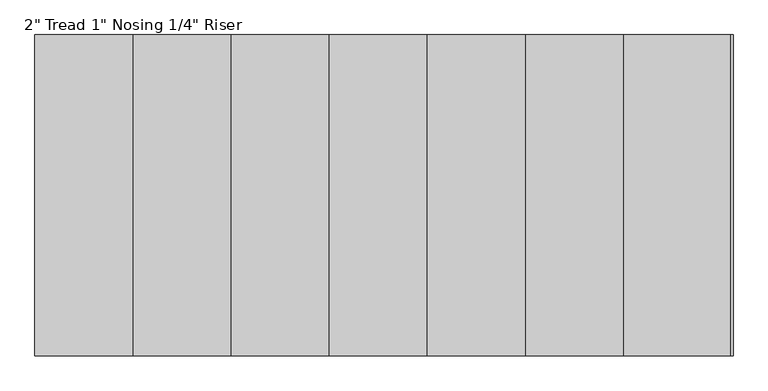
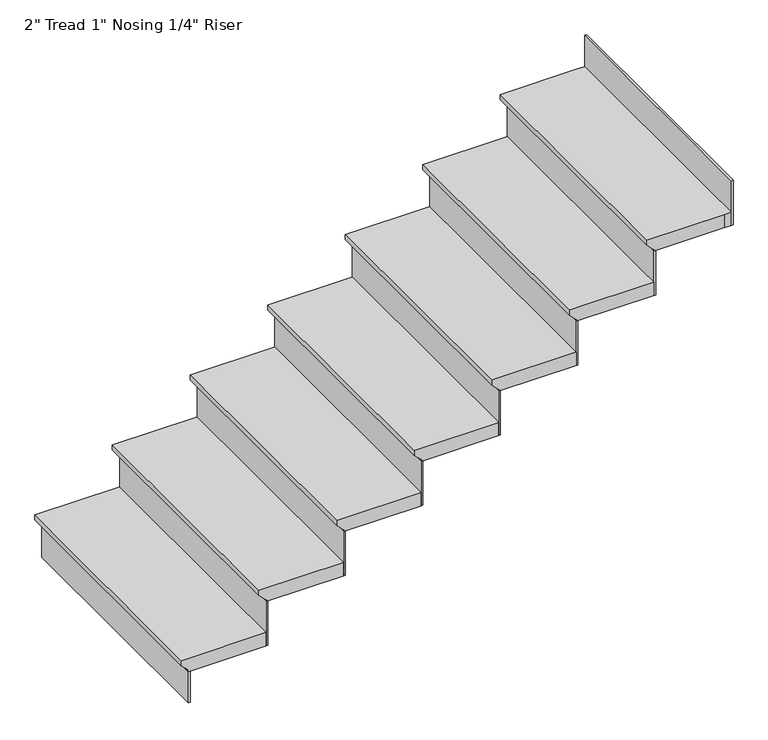
"""IFC4 building model written with IfcOpenShell, lengths in millimetres: stair flight geometry."""

from ifc_helpers import new_model, si_unit, origin, place, context, project, spatial, faceted_brep, source, transform, mapped, element, save


def stair_flight_171342da(model_context):
    return source(origin(), model_context, "Body", "Brep", [
        faceted_brep([(-1404.564062, 2339.7857363, 3503.0833333), (-1404.564062, 2339.7857363, 3522.1333333), (-1404.564062, 3254.1857363, 3522.1333333), (-1404.564062, 3254.1857363, 3503.0833333), (-1379.164062, 2339.7857363, 3477.6833333), (-1379.164062, 3254.1857363, 3477.6833333), (-1099.764062, 2339.7857363, 3522.1333333), (-1099.764062, 3254.1857363, 3522.1333333), (-1379.164062, 3254.1857363, 3471.3333333), (-1099.764062, 3254.1857363, 3471.3333333), (-1099.764062, 2339.7857363, 3471.3333333), (-1379.164062, 2339.7857363, 3471.3333333)], [[[0, 1, 2, 3]], [[4, 0, 3, 5]], [[2, 1, 6, 7]], [[8, 9, 10, 11]], [[2, 7, 9, 8, 5, 3]], [[8, 11, 4, 5]], [[6, 1, 0, 4, 11, 10]], [[7, 6, 10, 9]]]),
        faceted_brep([(-1379.164062, 2339.7857363, 3471.3333333), (-1379.164062, 2339.7857363, 3352.8), (-1372.814062, 2339.7857363, 3352.8), (-1372.814062, 2339.7857363, 3471.3333333), (-1379.164062, 3254.1857363, 3471.3333333), (-1372.814062, 3254.1857363, 3471.3333333), (-1372.814062, 3254.1857363, 3352.8), (-1379.164062, 3254.1857363, 3352.8)], [[[0, 1, 2, 3]], [[4, 5, 6, 7]], [[1, 0, 4, 7]], [[2, 1, 7, 6]], [[3, 2, 6, 5]], [[0, 3, 5, 4]]]),
        faceted_brep([(-1099.764062, 2339.7857363, 3640.6666667), (-1099.764062, 2339.7857363, 3471.3333333), (-1093.414062, 2339.7857363, 3471.3333333), (-1093.414062, 2339.7857363, 3640.6666667), (-1099.764062, 3254.1857363, 3640.6666667), (-1093.414062, 3254.1857363, 3640.6666667), (-1093.414062, 3254.1857363, 3471.3333333), (-1099.764062, 3254.1857363, 3471.3333333)], [[[0, 1, 2, 3]], [[4, 5, 6, 7]], [[1, 0, 4, 7]], [[2, 1, 7, 6]], [[3, 2, 6, 5]], [[0, 3, 5, 4]]]),
        faceted_brep([(-1125.164062, 3254.1857363, 3691.4666667), (-1125.164062, 2339.7857363, 3691.4666667), (-820.364062, 2339.7857363, 3691.4666667), (-820.364062, 3254.1857363, 3691.4666667), (-1099.764062, 3254.1857363, 3640.6666667), (-820.364062, 3254.1857363, 3640.6666667), (-820.364062, 2339.7857363, 3640.6666667), (-1099.764062, 2339.7857363, 3640.6666667), (-1099.764062, 3254.1857363, 3647.0166667), (-1125.164062, 3254.1857363, 3672.4166667), (-1099.764062, 2339.7857363, 3647.0166667), (-1125.164062, 2339.7857363, 3672.4166667)], [[[0, 1, 2, 3]], [[4, 5, 6, 7]], [[0, 3, 5, 4, 8, 9]], [[4, 7, 10, 8]], [[2, 1, 11, 10, 7, 6]], [[3, 2, 6, 5]], [[11, 1, 0, 9]], [[10, 11, 9, 8]]]),
        faceted_brep([(-820.364062, 2339.7857363, 3810.0), (-820.364062, 2339.7857363, 3640.6666667), (-814.014062, 2339.7857363, 3640.6666667), (-814.014062, 2339.7857363, 3810.0), (-820.364062, 3254.1857363, 3810.0), (-814.014062, 3254.1857363, 3810.0), (-814.014062, 3254.1857363, 3640.6666667), (-820.364062, 3254.1857363, 3640.6666667)], [[[0, 1, 2, 3]], [[4, 5, 6, 7]], [[1, 0, 4, 7]], [[2, 1, 7, 6]], [[3, 2, 6, 5]], [[0, 3, 5, 4]]]),
        faceted_brep([(-845.764062, 3254.1857363, 3860.8), (-845.764062, 2339.7857363, 3860.8), (-540.964062, 2339.7857363, 3860.8), (-540.964062, 3254.1857363, 3860.8), (-820.364062, 3254.1857363, 3810.0), (-540.964062, 3254.1857363, 3810.0), (-540.964062, 2339.7857363, 3810.0), (-820.364062, 2339.7857363, 3810.0), (-820.364062, 3254.1857363, 3816.35), (-845.764062, 3254.1857363, 3841.75), (-820.364062, 2339.7857363, 3816.35), (-845.764062, 2339.7857363, 3841.75)], [[[0, 1, 2, 3]], [[4, 5, 6, 7]], [[0, 3, 5, 4, 8, 9]], [[4, 7, 10, 8]], [[2, 1, 11, 10, 7, 6]], [[3, 2, 6, 5]], [[11, 1, 0, 9]], [[10, 11, 9, 8]]]),
        faceted_brep([(-540.964062, 2339.7857363, 3979.3333333), (-540.964062, 2339.7857363, 3810.0), (-534.614062, 2339.7857363, 3810.0), (-534.614062, 2339.7857363, 3979.3333333), (-540.964062, 3254.1857363, 3979.3333333), (-534.614062, 3254.1857363, 3979.3333333), (-534.614062, 3254.1857363, 3810.0), (-540.964062, 3254.1857363, 3810.0)], [[[0, 1, 2, 3]], [[4, 5, 6, 7]], [[1, 0, 4, 7]], [[2, 1, 7, 6]], [[3, 2, 6, 5]], [[0, 3, 5, 4]]]),
        faceted_brep([(-566.364062, 3254.1857363, 4030.1333333), (-566.364062, 2339.7857363, 4030.1333333), (-261.564062, 2339.7857363, 4030.1333333), (-261.564062, 3254.1857363, 4030.1333333), (-540.964062, 3254.1857363, 3979.3333333), (-261.564062, 3254.1857363, 3979.3333333), (-261.564062, 2339.7857363, 3979.3333333), (-540.964062, 2339.7857363, 3979.3333333), (-540.964062, 3254.1857363, 3985.6833333), (-566.364062, 3254.1857363, 4011.0833333), (-540.964062, 2339.7857363, 3985.6833333), (-566.364062, 2339.7857363, 4011.0833333)], [[[0, 1, 2, 3]], [[4, 5, 6, 7]], [[0, 3, 5, 4, 8, 9]], [[4, 7, 10, 8]], [[2, 1, 11, 10, 7, 6]], [[3, 2, 6, 5]], [[11, 1, 0, 9]], [[10, 11, 9, 8]]]),
        faceted_brep([(-261.564062, 2339.7857363, 4148.6666667), (-261.564062, 2339.7857363, 3979.3333333), (-255.214062, 2339.7857363, 3979.3333333), (-255.214062, 2339.7857363, 4148.6666667), (-261.564062, 3254.1857363, 4148.6666667), (-255.214062, 3254.1857363, 4148.6666667), (-255.214062, 3254.1857363, 3979.3333333), (-261.564062, 3254.1857363, 3979.3333333)], [[[0, 1, 2, 3]], [[4, 5, 6, 7]], [[1, 0, 4, 7]], [[2, 1, 7, 6]], [[3, 2, 6, 5]], [[0, 3, 5, 4]]]),
        faceted_brep([(-286.964062, 3254.1857363, 4199.4666667), (-286.964062, 2339.7857363, 4199.4666667), (17.835938, 2339.7857363, 4199.4666667), (17.835938, 3254.1857363, 4199.4666667), (-261.564062, 3254.1857363, 4148.6666667), (17.835938, 3254.1857363, 4148.6666667), (17.835938, 2339.7857363, 4148.6666667), (-261.564062, 2339.7857363, 4148.6666667), (-261.564062, 3254.1857363, 4155.0166667), (-286.964062, 3254.1857363, 4180.4166667), (-261.564062, 2339.7857363, 4155.0166667), (-286.964062, 2339.7857363, 4180.4166667)], [[[0, 1, 2, 3]], [[4, 5, 6, 7]], [[0, 3, 5, 4, 8, 9]], [[4, 7, 10, 8]], [[2, 1, 11, 10, 7, 6]], [[3, 2, 6, 5]], [[11, 1, 0, 9]], [[10, 11, 9, 8]]]),
        faceted_brep([(17.835938, 2339.7857363, 4318.0), (17.835938, 2339.7857363, 4148.6666667), (24.185938, 2339.7857363, 4148.6666667), (24.185938, 2339.7857363, 4318.0), (17.835938, 3254.1857363, 4318.0), (24.185938, 3254.1857363, 4318.0), (24.185938, 3254.1857363, 4148.6666667), (17.835938, 3254.1857363, 4148.6666667)], [[[0, 1, 2, 3]], [[4, 5, 6, 7]], [[1, 0, 4, 7]], [[2, 1, 7, 6]], [[3, 2, 6, 5]], [[0, 3, 5, 4]]]),
        faceted_brep([(-7.564062, 3254.1857363, 4368.8), (-7.564062, 2339.7857363, 4368.8), (297.235938, 2339.7857363, 4368.8), (297.235938, 3254.1857363, 4368.8), (17.835938, 3254.1857363, 4318.0), (297.235938, 3254.1857363, 4318.0), (297.235938, 2339.7857363, 4318.0), (17.835938, 2339.7857363, 4318.0), (17.835938, 3254.1857363, 4324.35), (-7.564062, 3254.1857363, 4349.75), (17.835938, 2339.7857363, 4324.35), (-7.564062, 2339.7857363, 4349.75)], [[[0, 1, 2, 3]], [[4, 5, 6, 7]], [[0, 3, 5, 4, 8, 9]], [[4, 7, 10, 8]], [[2, 1, 11, 10, 7, 6]], [[3, 2, 6, 5]], [[11, 1, 0, 9]], [[10, 11, 9, 8]]]),
        faceted_brep([(576.635938, 2339.7857363, 4656.6666667), (576.635938, 2339.7857363, 4487.3333333), (582.985938, 2339.7857363, 4487.3333333), (582.985938, 2339.7857363, 4656.6666667), (576.635938, 3254.1857363, 4656.6666667), (582.985938, 3254.1857363, 4656.6666667), (582.985938, 3254.1857363, 4487.3333333), (576.635938, 3254.1857363, 4487.3333333)], [[[0, 1, 2, 3]], [[4, 5, 6, 7]], [[1, 0, 4, 7]], [[2, 1, 7, 6]], [[3, 2, 6, 5]], [[0, 3, 5, 4]]]),
        faceted_brep([(297.235938, 2339.7857363, 4487.3333333), (297.235938, 2339.7857363, 4318.0), (303.585938, 2339.7857363, 4318.0), (303.585938, 2339.7857363, 4487.3333333), (297.235938, 3254.1857363, 4487.3333333), (303.585938, 3254.1857363, 4487.3333333), (303.585938, 3254.1857363, 4318.0), (297.235938, 3254.1857363, 4318.0)], [[[0, 1, 2, 3]], [[4, 5, 6, 7]], [[1, 0, 4, 7]], [[2, 1, 7, 6]], [[3, 2, 6, 5]], [[0, 3, 5, 4]]]),
        faceted_brep([(576.635938, 3254.1857363, 4538.1333333), (551.235938, 3254.1857363, 4538.1333333), (271.835938, 3254.1857363, 4538.1333333), (271.835938, 2339.7857363, 4538.1333333), (551.235938, 2339.7857363, 4538.1333333), (576.635938, 2339.7857363, 4538.1333333), (551.235938, 3254.1857363, 4487.3333333), (576.635938, 3254.1857363, 4487.3333333), (576.635938, 2339.7857363, 4487.3333333), (551.235938, 2339.7857363, 4487.3333333), (297.235938, 2339.7857363, 4487.3333333), (297.235938, 3254.1857363, 4487.3333333), (297.235938, 3254.1857363, 4493.6833333), (271.835938, 3254.1857363, 4519.0833333), (297.235938, 2339.7857363, 4493.6833333), (271.835938, 2339.7857363, 4519.0833333)], [[[0, 1, 2, 3, 4, 5]], [[6, 7, 8, 9, 10, 11]], [[1, 0, 7, 6]], [[2, 1, 6, 11, 12, 13]], [[11, 10, 14, 12]], [[4, 3, 15, 14, 10, 9]], [[5, 4, 9, 8]], [[0, 5, 8, 7]], [[15, 3, 2, 13]], [[14, 15, 13, 12]]]),
    ])


if __name__ == "__main__":
    model = new_model("IFC4")
    model_context = context("Model", 3, world=origin())
    ifc_project = project(units=[si_unit("LENGTHUNIT", "METRE", prefix="MILLI")], contexts=[model_context])
    site = spatial("IfcSite", under=ifc_project)
    building = spatial("IfcBuilding", under=site)
    placement = place(None, origin())
    stair_flight_shape = stair_flight_171342da(model_context)
    element("IfcStairFlight", 1, ObjectType="2\" Tread 1\" Nosing 1/4\" Riser", at=placement, inside=building, context=model_context, shape_type="MappedRepresentation", body=[
        mapped(stair_flight_shape, transform((0.0, 0.0, 0.0), x_axis=(1.0, 0.0, 0.0), y_axis=(0.0, 1.0, 0.0), z_axis=(0.0, 0.0, 1.0))),
    ])
    save(model, "model.ifc")

# Revit data of these elements
# Element 1 (IfcStairFlight, "2\" Tread 1\" Nosing 1/4\" Riser")
#   Materials on its faces: "BURGUNDY COLOUR"
# Materials
#   "BURGUNDY COLOUR": class "Generic", colour RGB 120 120 120, transparency 0, Cost = 0
